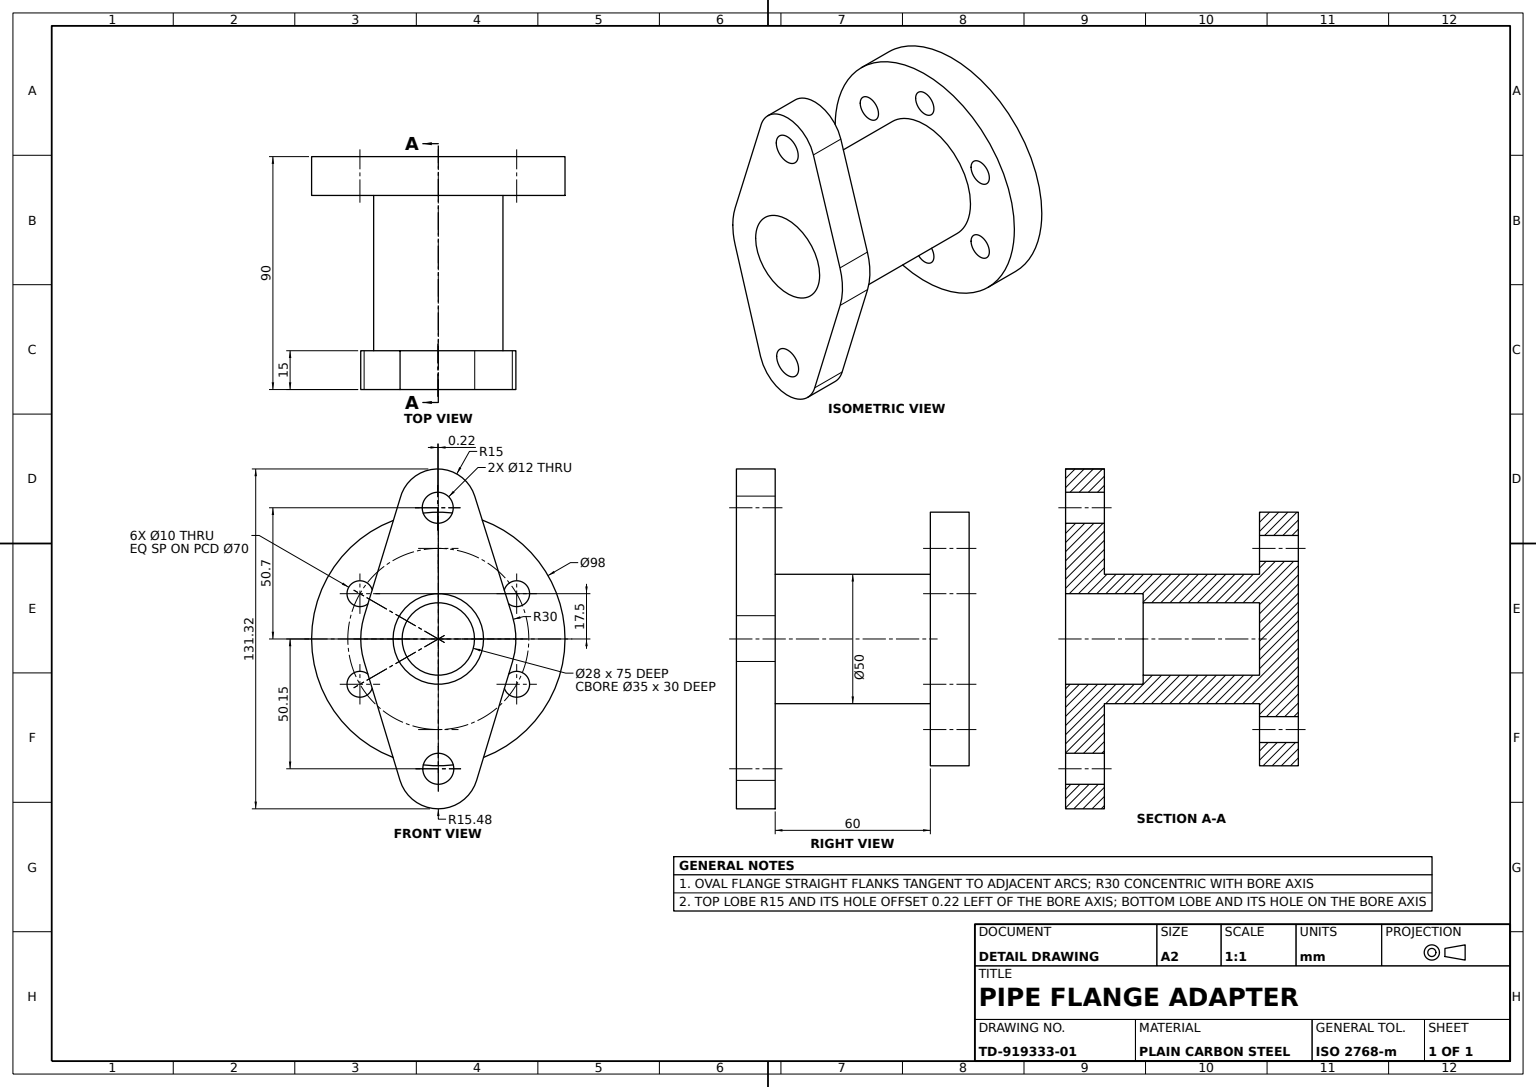
SolidWorks part; units mm, degrees
material "Plain Carbon Steel"
ref_plane "Front Plane" through (0, 0, 0) normal (0, 0, 1) x (1, 0, 0)
ref_plane "Top Plane" through (0, 0, 0) normal (0, 1, 0) x (1, 0, 0)
ref_plane "Right Plane" through (0, 0, 0) normal (1, 0, 0) x (0, 0, -1)
sketch "Round Flange Sketch" plane through (0, 0, 0) normal (0, 0, 1) x (1, 0, 0)
  circle A0 centre (0, 0) radius 49
  dimension "D1" = 98
  dimension "D2" = 98
extrude "Round Flange Ø98" add sketch "Round Flange Sketch" along normal blind 15
sketch "Round Flange Holes Sketch" plane through (0, 0, 15) normal (0, 0, 1) x (1, 0, 0)
  circle A1 centre (0, 35) radius 5
  circle A2 centre (30.3109, 17.5) radius 5
  circle A3 centre (30.3109, -17.5) radius 5
  circle A4 centre (0, -35) radius 5
  circle A5 centre (-30.3109, -17.5) radius 5
  circle A6 centre (-30.3109, 17.5) radius 5
  circle A7 centre (0, 0) radius 49 construction
  dimension "D1" = 10
  dimension "D2" = 10
  dimension "D4" = 30.3109
  dimension "D5" = 30.3109
  dimension "D6" = 17.5
  dimension "D3" = 6
extrude "Round Flange Holes 6xØ10" cut sketch "Round Flange Holes Sketch" against normal blind 15
sketch "Sleeve Sketch" plane through (0, 0, 15) normal (0, 0, 1) x (1, 0, 0)
  circle A0 centre (0, 0) radius 25
  dimension "D1" = 50
  dimension "D2" = 50
extrude "Sleeve Ø50" add sketch "Sleeve Sketch" along normal blind 60
sketch "Oval Flange Sketch" plane through (0, 0, 75) normal (0, 0, 1) x (1, 0, 0)
  line L0 (-14.8125, -54.6338) -> (-28.7144, -8.6882)
  line L2 (-14.7865, 54.2638) -> (-28.6902, 8.7678)
  line L3 (14.0839, 55.2008) -> (28.6173, 9.0027)
  line L4 (14.8125, -54.6338) -> (28.7144, -8.6882)
  arc A0 (-28.6902, 8.7678) -> (-28.7144, -8.6882) centre (0, 0) ccw
  arc A1 (14.0839, 55.2008) -> (-14.7865, 54.2638) centre (-0.2205, 50.7008) ccw
  arc A2 (-14.8125, -54.6338) -> (14.8125, -54.6338) centre (0, -50.1519) ccw
  arc A3 (28.7144, -8.6882) -> (28.6173, 9.0027) centre (0, 0) ccw
  circle A4 centre (0, 0) radius 25 construction
  dimension "D1" = 60
  dimension "D2" = 29.991
  dimension "D3" = 30.9514
  dimension "D4" = 30
  dimension "D5" = 14.9955
  dimension "D6" = 15.4757
  dimension "D7" = 14.0839
  dimension "D8" = 14.8125
  dimension "D9" = 28.6173
  dimension "D10" = 14.7865
extrude "Oval Flange" add sketch "Oval Flange Sketch" along normal blind 15
sketch "Oval Flange Holes Sketch" plane through (0, 0, 90) normal (0, 0, 1) x (1, 0, 0)
  circle A0 centre (-0.2205, 50.7008) radius 6
  circle A1 centre (0, -50.1519) radius 6
  dimension "D1" = 12
  dimension "D2" = 12
  dimension "D3" = 12
extrude "Oval Flange Holes 2xØ12" cut sketch "Oval Flange Holes Sketch" against normal blind 15
sketch "Counterbore Sketch" plane through (0, 0, 90) normal (0, 0, 1) x (1, 0, 0)
  circle A0 centre (0, 0) radius 17.5
  dimension "D1" = 35
  dimension "D2" = 35
extrude "Counterbore Ø35" cut sketch "Counterbore Sketch" against normal blind 30
sketch "Bore Sketch" plane through (0, 0, 60) normal (0, 0, 1) x (1, 0, 0)
  circle A0 centre (0, 0) radius 14
  dimension "D1" = 28
  dimension "D2" = 28
extrude "Bore Ø28" cut sketch "Bore Sketch" against normal blind 45
